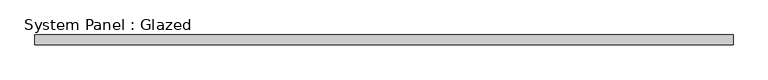
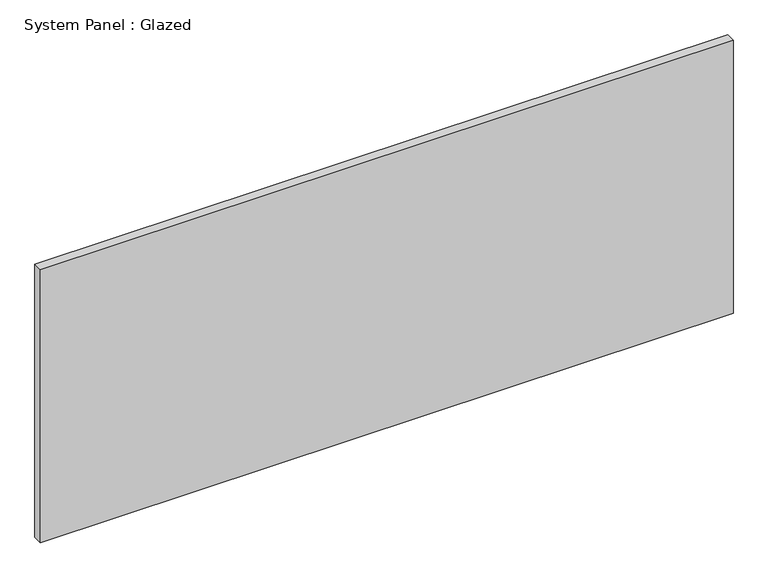
"""IFC4 building model written with IfcOpenShell, lengths in millimetres: plate geometry, System Panel : Glazed."""

from ifc_helpers import new_model, si_unit, origin, origin_with_axes, place, context, project, spatial, polyline, outline, extrude, source, transform, mapped, element, save


def system_panel_glazed_22be659e(model_context):
    return source(origin(), model_context, "Body", "SweptSolid", [
        extrude(outline(polyline([(914.4, 19.05), (-914.4, 19.05), (-914.4, 44.45), (914.4, 44.45), (914.4, 19.05)])), origin_with_axes(), (0.0, 0.0, 1.0), 762.0),
    ])


if __name__ == "__main__":
    model = new_model("IFC4")
    model_context = context("Model", 3, world=origin())
    ifc_project = project(units=[si_unit("LENGTHUNIT", "METRE", prefix="MILLI")], contexts=[model_context])
    site = spatial("IfcSite", under=ifc_project)
    building = spatial("IfcBuilding", under=site)
    placement = place(None, origin())
    system_panel_glazed_shape = system_panel_glazed_22be659e(model_context)
    element("IfcPlate", 1, ObjectType="System Panel : Glazed", at=placement, inside=building, context=model_context, shape_type="MappedRepresentation", body=[
        mapped(system_panel_glazed_shape, transform((0.0, 0.0, 0.0), x_axis=(1.0, 0.0, 0.0), y_axis=(0.0, 1.0, 0.0), z_axis=(0.0, 0.0, 1.0))),
    ])
    save(model, "model.ifc")

# Revit data of these elements
# Type "System Panel : Glazed"
#   Construction Type Id = "GSP4R"
#   Analytic Construction = "1/8 in Pilkington single glazing"
#   Visual Light Transmittance = 0.9
#   Solar Heat Gain Coefficient = 0.86
#   Heat Transfer Coefficient (U) = 1.18115 BTU/(h·ft²·°F)
# Element 1 (IfcPlate, "System Panel : Glazed")
#   Materials on its faces: "Glass"
# Materials
#   "Glass": class "Glass", colour RGB 0 128 192, transparency 0.75, Description = "Soda Lime Glass", Cost = 0
